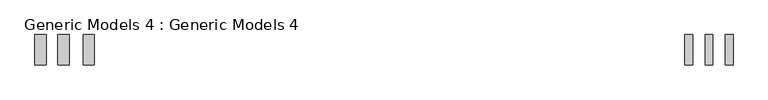
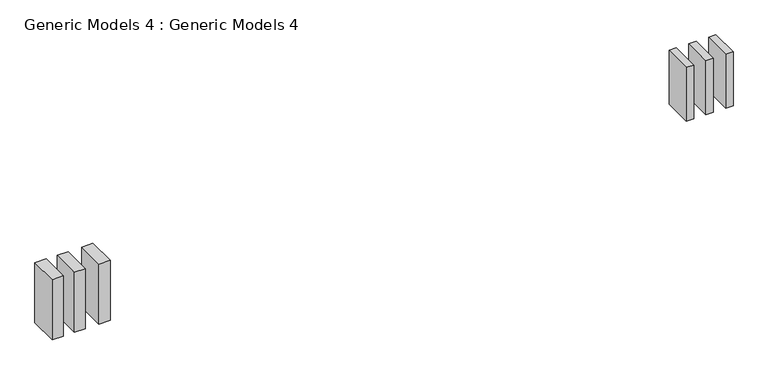
"""IFC4 building model written with IfcOpenShell, lengths in millimetres: proxy geometry, Generic Models 4 : Generic Models 4."""

from ifc_helpers import new_model, si_unit, frame, origin, place, context, project, spatial, polyline, outline, extrude, source, transform, mapped, element, save


def generic_models_4_generic_models_4_efd0a726(model_context):
    return source(origin(), model_context, "Body", "SweptSolid", [
        extrude(outline(polyline([(2575.1589785, -6867.8109248), (2498.9589785, -6867.8109248), (2498.9589785, -6563.0109248), (2575.1589785, -6563.0109248), (2575.1589785, -6867.8109248)])), frame((0.0, 0.0, 854.2482387), z_axis=(0.0, 0.0, 1.0), x_axis=(1.0, 0.0, 0.0)), (0.0, 0.0, 1.0), 584.2),
        extrude(outline(polyline([(2371.9589785, -6867.8109248), (2295.7589785, -6867.8109248), (2295.7589785, -6563.0109248), (2371.9589785, -6563.0109248), (2371.9589785, -6867.8109248)])), frame((0.0, 0.0, 854.2482387), z_axis=(0.0, 0.0, 1.0), x_axis=(1.0, 0.0, 0.0)), (0.0, 0.0, 1.0), 584.2),
        extrude(outline(polyline([(2168.7589785, -6867.8109248), (2092.5589785, -6867.8109248), (2092.5589785, -6563.0109248), (2168.7589785, -6563.0109248), (2168.7589785, -6867.8109248)])), frame((0.0, 0.0, 854.2482387), z_axis=(0.0, 0.0, 1.0), x_axis=(1.0, 0.0, 0.0)), (0.0, 0.0, 1.0), 584.2),
        extrude(outline(polyline([(-4312.8589614, -6867.8109248), (-4427.1589614, -6867.8109248), (-4427.1589614, -6563.0109248), (-4312.8589614, -6563.0109248), (-4312.8589614, -6867.8109248)])), frame((0.0, 0.0, 762.0), z_axis=(0.0, 0.0, 1.0), x_axis=(1.0, 0.0, 0.0)), (0.0, 0.0, 1.0), 652.6369184),
        extrude(outline(polyline([(-4084.2589614, -6867.8109248), (-4198.5589614, -6867.8109248), (-4198.5589614, -6563.0109248), (-4084.2589614, -6563.0109248), (-4084.2589614, -6867.8109248)])), frame((0.0, 0.0, 762.0), z_axis=(0.0, 0.0, 1.0), x_axis=(1.0, 0.0, 0.0)), (0.0, 0.0, 1.0), 652.6369184),
        extrude(outline(polyline([(-3830.2589614, -6867.8109248), (-3944.5589614, -6867.8109248), (-3944.5589614, -6563.0109248), (-3830.2589614, -6563.0109248), (-3830.2589614, -6867.8109248)])), frame((0.0, 0.0, 762.0), z_axis=(0.0, 0.0, 1.0), x_axis=(1.0, 0.0, 0.0)), (0.0, 0.0, 1.0), 652.6369184),
    ])


if __name__ == "__main__":
    model = new_model("IFC4")
    model_context = context("Model", 3, world=origin())
    ifc_project = project(units=[si_unit("LENGTHUNIT", "METRE", prefix="MILLI")], contexts=[model_context])
    site = spatial("IfcSite", under=ifc_project)
    building = spatial("IfcBuilding", under=site)
    placement = place(None, origin())
    generic_models_4_generic_models_4_shape = generic_models_4_generic_models_4_efd0a726(model_context)
    element("IfcBuildingElementProxy", 1, Name="Generic Models 4 : Generic Models 4", ObjectType="Generic Models 4 : Generic Models 4", at=placement, inside=building, context=model_context, shape_type="MappedRepresentation", body=[
        mapped(generic_models_4_generic_models_4_shape, transform((0.0, 0.0, 0.0), x_axis=(1.0, 0.0, 0.0), y_axis=(0.0, 1.0, 0.0), z_axis=(0.0, 0.0, 1.0))),
    ])
    save(model, "model.ifc")

# Revit data of these elements
# Element 1 (IfcBuildingElementProxy, "Generic Models 4 : Generic Models 4")
#   Materials on its faces: "Parking Stripe"
# Materials
#   "Parking Stripe": class "Paint", colour RGB 250 250 91, transparency 0, Cost = 0
